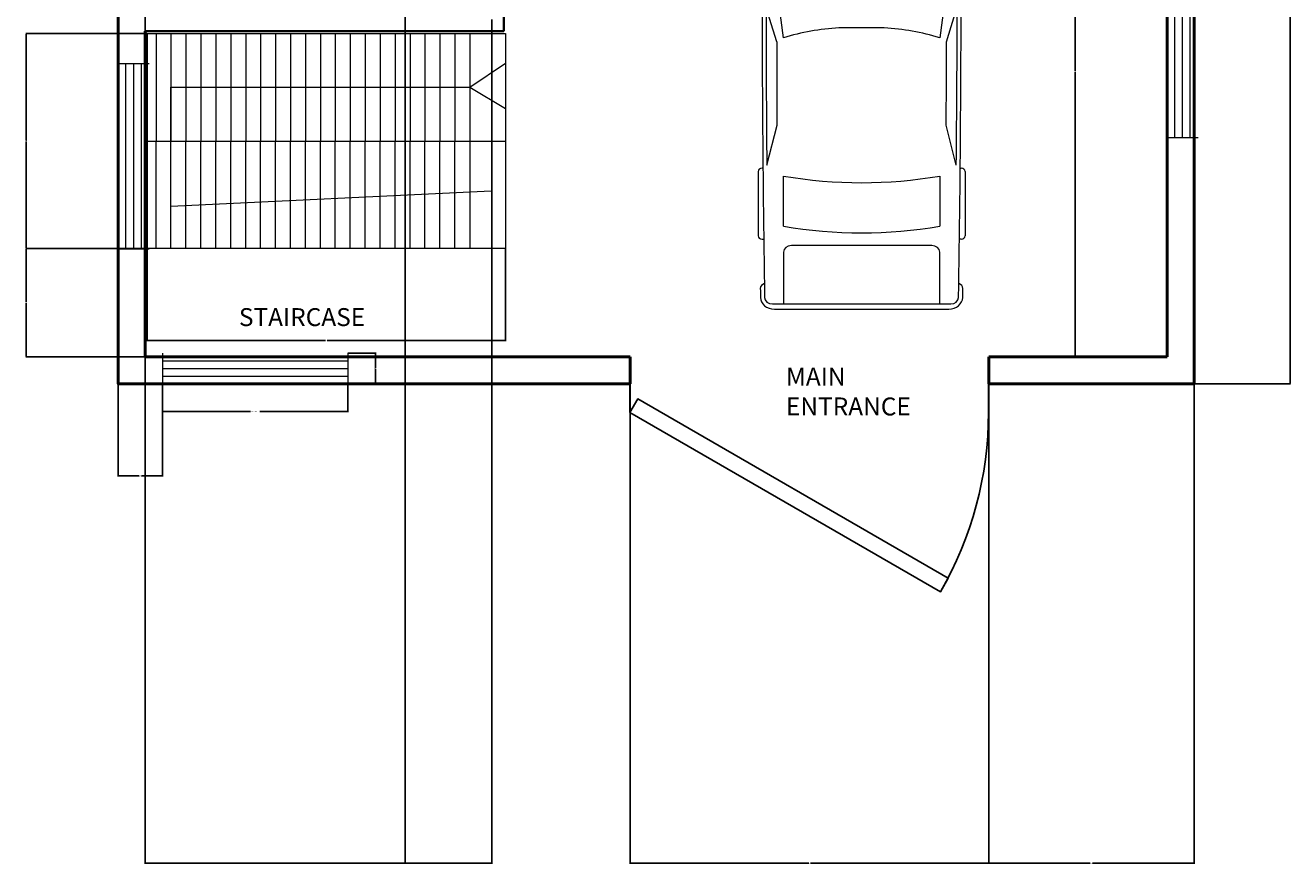
# Model space of a CAD drawing. Units: feet. Extents: x 3746 to 4170, y 1475 to 2148.
# Tile 1 of 5: x 3746 to 4170, y 1475 to 1755. Entities that reach past the tile are written whole.
import ezdxf

# ---------------------------------------------------------------- set-up
doc = ezdxf.new("R2010")
doc.units = ezdxf.units.FT
for name, color, linetype, lineweight in [('A-ANNO-DIMS', 2, 'Continuous', 18), ('A-AREA-IDEN', 7, 'Continuous', 25), ('A-FLOR-STRS', 7, 'Continuous', 18), ('A-GLAZ', 91, 'Continuous', 18), ('CAR', 20, 'Continuous', 13), ('DOOR', 135, 'Continuous', 25), ('INWER WALL', 30, 'Continuous', 35), ('OUTER WALL', 31, 'Continuous', 50)]:
    doc.layers.add(name, color=color, linetype=linetype, lineweight=lineweight)
doc.styles.get("Standard").update_dxf_attribs({"font": 'arial.ttf'})
doc.dimstyles.get("Standard").update_dxf_attribs({"dimtxt": 0.18, "dimasz": 0.18, "dimexe": 0.18, "dimexo": 0.0625, "dimgap": 0.09, "dimtad": 0, "dimtih": 1, "dimtoh": 1, "dimdec": 4, "dimzin": 0, "dimdsep": 46, "dimtxsty": 'Standard', "dimcen": 0.09, "dimadec": 0, "dimazin": 0, "dimtfac": 1, "dimtdec": 4, "dimtofl": 0, "dimtmove": 0, "dimatfit": 3, "dimfxl": 1, "dimtolj": 1, "dimtzin": 0, "dimarcsym": 0})

# ---------------------------------------------------------------- blocks, each defined once
blk = doc.blocks.new('*U12')
for p, q in [((46.55, 38.89), (22.35, 38.89)), ((136.7, 38.89), (160.9, 38.89)), ((21.1, 37.41), (21.1, 36.83)), ((47.8, 37.39), (47.8, 37.41)), ((87.99, 31.87), (74.76, 35.92)), ((134.31, 35.6), (119.29, 31.78)), ((135.45, 37.07), (135.45, 37.41)), ((162.15, 37.41), (162.15, 36.77)), ((186.47, -33.5), (186.47, 33.5)), ((70.03, 31.54), (86.41, 29.35)), ((138.42, 29.35), (157.25, 29.35)), ((186.47, 29.35), (167.01, 29.35)), ((188.4, -32.76), (188.4, 32.76)), ((164.52, 26.39), (164.52, -26.39)), ((32.27, 11.63), (36.13, 17.17)), ((36.13, 17.17), (50.94, 17.17)), ((32.12, 9.51), (32.12, 11.15)), ((58.92, -10.77), (58.92, 10.77)), ((66.55, -10.53), (66.55, 10.53)), ((186.47, -10.53), (186.47, 10.53)), ((3.27, 6.13), (0.1, 0.41)), ((29.77, 9.51), (51.68, 9.51)), ((82.74, 8.5), (82.74, -8.5)), ((0, 0), (51.68, 0)), ((0.1, -0.41), (3.27, -6.13)), ((29.77, -9.51), (51.68, -9.51)), ((32.12, -9.51), (32.12, -11.15)), ((32.27, -11.63), (36.13, -17.17)), ((36.13, -17.17), (50.94, -17.17)), ((86.41, -29.35), (70.03, -31.54)), ((87.99, -31.87), (74.76, -35.92)), ((134.31, -35.6), (119.29, -31.78)), ((157.25, -29.35), (138.42, -29.35)), ((167.01, -29.35), (186.47, -29.35)), ((21.1, -37.41), (21.1, -36.83)), ((47.8, -37.39), (47.8, -37.41)), ((135.45, -37.07), (135.45, -37.41)), ((162.15, -37.41), (162.15, -36.77)), ((46.55, -38.89), (22.35, -38.89)), ((136.7, -38.89), (160.9, -38.89))]:
    blk.add_line(p, q)
for centre, major_axis, ratio, start_param, end_param in [((22.35, 37.41), (0, -1.48), 0.842304, 3.141593, 4.712389), ((46.55, 37.41), (0, 1.48), 0.842304, -1.570796, 0), ((136.7, 37.41), (0, -1.48), 0.842304, 3.141593, 4.712389), ((160.9, 37.41), (0, 1.48), 0.842304, -1.570796, 0), ((180.63, 35.84), (0, 2.22), 0.842304, -0.013017, 1.249894), ((64.48, -10556.36), (0, 10595.31), 0.842304, -0.013397, -0.013017), ((266.03, -27.52), (0, 313.31), 0.842304, 1.367076, 1.39176), ((41.19, -490.86), (0, 528.23), 0.842304, 0.00281, 0.075598), ((64.48, -10555.62), (0, 10593.03), 0.842304, -0.013397, 0.002797), ((64.48, -10555.62), (0, -10591.55), 0.842304, 3.133765, 3.140441), ((183.98, 33.5), (0, -2.96), 0.842304, 1.570796, 3.128196), ((183.98, 32.76), (0, -5.25), 0.842304, 1.570796, 3.128196), ((37.47, -593.96), (0, -623.33), 0.842304, 3.096046, 3.200911), ((134.4, 5.39), (0, -89.78), 0.842304, 4.449482, 4.652344), ((135.29, 5.39), (0, 81.77), 0.842304, 1.245306, 1.50788), ((149.6, 2.8), (0, -79.58), 0.842304, 4.372215, 4.640744), ((95.79, -3666.35), (0, -3698.24), 0.842304, 3.134049, 3.144098), ((17.08, 0), (0, 147.02), 0.842304, 4.511394, 4.913384), ((35.91, 0), (0, 147.02), 0.842304, 4.511394, 4.913384), ((167.01, 26.39), (0, 2.96), 0.842304, 0, 1.570796), ((259.18, -27.52), (0, -305.3), 0.842304, 4.528606, 4.561838), ((-204.49, 52.4), (0, -250.96), 0.842304, 1.385369, 1.434372), ((13.04, 17.01), (0, 27.42), 0.842304, 4.435146, 4.718221), ((14.2, 17.01), (0, 27.42), 0.842304, 4.435146, 4.718221), ((50.79, 13.34), (6.34, -0.36), 0.603834, -1.395552, 1.581315), ((32.75, 11.15), (0, 0.74), 0.842304, 0.879714, 1.570796), ((29.77, -46.66), (0, 56.17), 0.842304, 0, 0.590319), ((0.62, 0), (0, -0.74), 0.842304, 4.131459, 5.293319), ((29.77, 46.66), (0, 56.17), 0.842304, 2.551274, 3.141593), ((-204.49, -52.4), (0, 250.96), 0.842304, -1.434372, -1.385369), ((13.04, -17.01), (0, -27.42), 0.842304, 1.564964, 1.848039), ((14.2, -17.01), (0, -27.42), 0.842304, 1.564964, 1.848039), ((149.6, -2.8), (0, -79.58), 0.842304, -1.499151, -1.230623), ((32.75, -11.15), (0, -0.74), 0.842304, 4.712389, 5.403472), ((134.4, -5.39), (0, -89.78), 0.842304, -1.510751, -1.307889), ((135.29, -5.39), (0, -81.77), 0.842304, -1.50788, -1.245306), ((259.18, 27.52), (0, 305.3), 0.842304, 1.721348, 1.754579), ((266.03, 27.52), (0, 313.31), 0.842304, 1.749832, 1.774517), ((37.47, 593.96), (0, -623.33), 0.842304, -0.059319, 0.045547), ((167.01, -26.39), (0, -2.96), 0.842304, 4.712389, 6.283185), ((95.79, 3666.35), (0, -3698.24), 0.842304, -0.002505, 0.007544), ((183.98, -32.76), (0, -5.25), 0.842304, 0.013397, 1.570796), ((41.19, 490.86), (0, -528.23), 0.842304, -0.075598, -0.00281), ((22.35, -37.41), (0, 1.48), 0.842304, 1.570796, 3.141593), ((64.48, 10555.62), (0, 10593.03), 0.842304, 3.138796, 3.15499), ((46.55, -37.41), (0, -1.48), 0.842304, 0, 1.570796), ((64.48, 10555.62), (0, -10591.55), 0.842304, 0.001152, 0.007828), ((136.7, -37.41), (0, -1.48), 0.842304, -1.570796, 0), ((160.9, -37.41), (0, 1.48), 0.842304, 3.141593, 4.712389), ((180.63, -35.84), (0, -2.22), 0.842304, -1.249894, 0.013017), ((64.48, 10556.36), (0, 10595.31), 0.842304, 3.15461, 3.15499), ((183.98, -33.5), (0, 2.96), 0.842304, 3.15499, 4.712389)]:
    blk.add_ellipse(centre, major_axis=major_axis, ratio=ratio, start_param=start_param, end_param=end_param)
at = {"extrusion": (0, 0, -1)}
blk.add_ellipse((50.79, -13.34), major_axis=(6.34, 0.36), ratio=0.603834, start_param=-1.395552, end_param=1.581315, dxfattribs=at)
blk = doc.blocks.new('*U3')
for p, q in [((0, 0), (0, 6)), ((40, 0), (40, 6))]:
    blk.add_line(p, q)
blk.add_lwpolyline([(0, 0), (34.64, -20), (35.52, -18.48), (0.87, 1.52)], close=True)
blk.add_arc((0, 0), 40, 330, 0)
blk = doc.blocks.new('Window - Wood Frame 36 in. Wide plan')
for p, q in [((0, 6), (0, 0)), ((36, 6), (36, 0)), ((0, 4.5), (36, 4.5)), ((0, 3), (36, 3)), ((0, 1.5), (36, 1.5))]:
    blk.add_line(p, q)
blk = doc.blocks.new('*D37')
at = {"layer": 'A-ANNO-DIMS', "color": 0, "lineweight": -2, "transparency": 16777216}
for p, q in [((3792.26, 1635.32), (3792.26, 1625.91)), ((3854.23, 1635.32), (3854.23, 1625.91)), ((3792.44, 1626.09), (3821.69, 1626.09)), ((3854.05, 1626.09), (3824.8, 1626.09))]:
    blk.add_line(p, q, dxfattribs=at)
at = {"layer": 'A-ANNO-DIMS', "color": 0, "transparency": 16777216}
for points in [[(3792.44, 1626.12), (3792.44, 1626.06), (3792.26, 1626.09)], [(3854.05, 1626.12), (3854.05, 1626.06), (3854.23, 1626.09)]]:
    blk.add_solid(points, dxfattribs=at)
at = {"layer": 'Defpoints', "color": 0, "transparency": 16777216}
for p in [(3792.26, 1635.38), (3854.23, 1635.38), (3854.23, 1626.09)]:
    blk.add_point(p, dxfattribs=at)
at = {"layer": 'A-ANNO-DIMS', "color": 0, "transparency": 16777216, "insert": (3823.24, 1626.09), "char_height": 0.18, "attachment_point": 5}
blk.add_mtext('\\A1;WOOD WINDOW 62 TYP.', dxfattribs=at)
blk = doc.blocks.new('*D38')
at = {"layer": 'A-ANNO-DIMS', "color": 0, "lineweight": -2, "transparency": 16777216}
for p, q in [((3854.29, 1645.71), (3863.7, 1645.71)), ((3863.52, 1645.53), (3863.52, 1640.73)), ((3863.52, 1635.56), (3863.52, 1640.36)), ((3854.29, 1635.38), (3863.7, 1635.38))]:
    blk.add_line(p, q, dxfattribs=at)
at = {"layer": 'A-ANNO-DIMS', "color": 0, "transparency": 16777216}
for points in [[(3863.49, 1645.53), (3863.55, 1645.53), (3863.52, 1645.71)], [(3863.49, 1635.56), (3863.55, 1635.56), (3863.52, 1635.38)]]:
    blk.add_solid(points, dxfattribs=at)
at = {"layer": 'Defpoints', "color": 0, "transparency": 16777216}
for p in [(3854.23, 1645.71), (3863.52, 1645.71), (3854.23, 1635.38)]:
    blk.add_point(p, dxfattribs=at)
at = {"layer": 'A-ANNO-DIMS', "color": 0, "transparency": 16777216, "insert": (3863.52, 1640.55), "char_height": 0.18, "attachment_point": 5}
blk.add_mtext('\\A1;10 TYP.', dxfattribs=at)
blk = doc.blocks.new('*D56')
at = {"layer": 'A-ANNO-DIMS', "color": 0, "lineweight": -2, "transparency": 16777216}
for p, q in [((4137.49, 2115.38), (4169.74, 2115.38)), ((4169.56, 2115.2), (4169.56, 1875.56)), ((4169.56, 1635.56), (4169.56, 1875.2)), ((4137.49, 1635.38), (4169.74, 1635.38))]:
    blk.add_line(p, q, dxfattribs=at)
at = {"layer": 'A-ANNO-DIMS', "color": 0, "transparency": 16777216}
for points in [[(4169.53, 2115.2), (4169.59, 2115.2), (4169.56, 2115.38)], [(4169.53, 1635.56), (4169.59, 1635.56), (4169.56, 1635.38)]]:
    blk.add_solid(points, dxfattribs=at)
at = {"layer": 'Defpoints', "color": 0, "transparency": 16777216}
for p in [(4137.43, 2115.38), (4137.43, 1635.38), (4169.56, 1635.38)]:
    blk.add_point(p, dxfattribs=at)
at = {"layer": 'A-ANNO-DIMS', "color": 0, "transparency": 16777216, "insert": (4169.56, 1875.38), "char_height": 0.18, "attachment_point": 5}
blk.add_mtext('\\A1;480', dxfattribs=at)
blk = doc.blocks.new('*D63')
at = {"layer": 'A-ANNO-DIMS', "color": 0, "lineweight": -2, "transparency": 16777216}
for p, q in [((3786.43, 1970.32), (3786.43, 1474.8)), ((3873.43, 1922.32), (3873.43, 1474.8)), ((3786.61, 1474.98), (3829.71, 1474.98)), ((3873.25, 1474.98), (3830.15, 1474.98))]:
    blk.add_line(p, q, dxfattribs=at)
at = {"layer": 'A-ANNO-DIMS', "color": 0, "transparency": 16777216}
for points in [[(3786.61, 1475.01), (3786.61, 1474.95), (3786.43, 1474.98)], [(3873.25, 1475.01), (3873.25, 1474.95), (3873.43, 1474.98)]]:
    blk.add_solid(points, dxfattribs=at)
at = {"layer": 'Defpoints', "color": 0, "transparency": 16777216}
for p in [(3786.43, 1970.38), (3873.43, 1922.38), (3873.43, 1474.98)]:
    blk.add_point(p, dxfattribs=at)
at = {"layer": 'A-ANNO-DIMS', "color": 0, "transparency": 16777216, "insert": (3829.93, 1474.98), "char_height": 0.18, "attachment_point": 5}
blk.add_mtext('\\A1;87', dxfattribs=at)
blk = doc.blocks.new('*D68')
at = {"layer": 'A-ANNO-DIMS', "color": 0, "lineweight": -2, "transparency": 16777216}
for p, q in [((3786.43, 1757.32), (3786.43, 1474.8)), ((3902.43, 1757.32), (3902.43, 1474.8)), ((3786.61, 1474.98), (3844.15, 1474.98)), ((3902.25, 1474.98), (3844.71, 1474.98))]:
    blk.add_line(p, q, dxfattribs=at)
at = {"layer": 'A-ANNO-DIMS', "color": 0, "transparency": 16777216}
for points in [[(3786.61, 1475.01), (3786.61, 1474.95), (3786.43, 1474.98)], [(3902.25, 1475.01), (3902.25, 1474.95), (3902.43, 1474.98)]]:
    blk.add_solid(points, dxfattribs=at)
at = {"layer": 'Defpoints', "color": 0, "transparency": 16777216}
for p in [(3786.43, 1757.38), (3902.43, 1757.38), (3902.43, 1474.98)]:
    blk.add_point(p, dxfattribs=at)
at = {"layer": 'A-ANNO-DIMS', "color": 0, "transparency": 16777216, "insert": (3844.43, 1474.98), "char_height": 0.18, "attachment_point": 5}
blk.add_mtext('\\A1;116', dxfattribs=at)
blk = doc.blocks.new('*D72')
at = {"layer": 'A-ANNO-DIMS', "color": 0, "lineweight": -2, "transparency": 16777216}
for p, q in [((4128.37, 1835.38), (4097.45, 1835.38)), ((4097.63, 1835.2), (4097.63, 1740.06)), ((4097.63, 1644.56), (4097.63, 1739.7)), ((4128.37, 1644.38), (4097.45, 1644.38))]:
    blk.add_line(p, q, dxfattribs=at)
at = {"layer": 'A-ANNO-DIMS', "color": 0, "transparency": 16777216}
for points in [[(4097.6, 1835.2), (4097.66, 1835.2), (4097.63, 1835.38)], [(4097.6, 1644.56), (4097.66, 1644.56), (4097.63, 1644.38)]]:
    blk.add_solid(points, dxfattribs=at)
at = {"layer": 'Defpoints', "color": 0, "transparency": 16777216}
for p in [(4097.63, 1835.38), (4128.43, 1835.38), (4128.43, 1644.38)]:
    blk.add_point(p, dxfattribs=at)
at = {"layer": 'A-ANNO-DIMS', "color": 0, "transparency": 16777216, "insert": (4097.63, 1739.88), "char_height": 0.18, "attachment_point": 5}
blk.add_mtext('\\A1;191', dxfattribs=at)
blk = doc.blocks.new('*D73')
at = {"layer": 'A-ANNO-DIMS', "color": 0, "lineweight": -2, "transparency": 16777216}
for p, q in [((3787, 1752.65), (3746.45, 1752.65)), ((3746.63, 1752.47), (3746.63, 1716.83)), ((3746.63, 1680.83), (3746.63, 1716.47)), ((3787, 1680.65), (3746.45, 1680.65))]:
    blk.add_line(p, q, dxfattribs=at)
at = {"layer": 'A-ANNO-DIMS', "color": 0, "transparency": 16777216}
for points in [[(3746.6, 1752.47), (3746.66, 1752.47), (3746.63, 1752.65)], [(3746.6, 1680.83), (3746.66, 1680.83), (3746.63, 1680.65)]]:
    blk.add_solid(points, dxfattribs=at)
at = {"layer": 'Defpoints', "color": 0, "transparency": 16777216}
for p in [(3787.06, 1752.65), (3746.63, 1680.65), (3787.06, 1680.65)]:
    blk.add_point(p, dxfattribs=at)
at = {"layer": 'A-ANNO-DIMS', "color": 0, "transparency": 16777216, "insert": (3746.63, 1716.65), "char_height": 0.18, "attachment_point": 5}
blk.add_mtext('\\A1;72', dxfattribs=at)
blk = doc.blocks.new('*D74')
at = {"layer": 'A-ANNO-DIMS', "color": 0, "lineweight": -2, "transparency": 16777216}
for p, q in [((3787, 1680.65), (3746.45, 1680.65)), ((3746.63, 1680.47), (3746.63, 1662.7)), ((3746.63, 1644.56), (3746.63, 1662.34)), ((3786.37, 1644.38), (3746.45, 1644.38))]:
    blk.add_line(p, q, dxfattribs=at)
at = {"layer": 'A-ANNO-DIMS', "color": 0, "transparency": 16777216}
for points in [[(3746.6, 1680.47), (3746.66, 1680.47), (3746.63, 1680.65)], [(3746.6, 1644.56), (3746.66, 1644.56), (3746.63, 1644.38)]]:
    blk.add_solid(points, dxfattribs=at)
at = {"layer": 'Defpoints', "color": 0, "transparency": 16777216}
for p in [(3787.06, 1680.65), (3746.63, 1644.38), (3786.43, 1644.38)]:
    blk.add_point(p, dxfattribs=at)
at = {"layer": 'A-ANNO-DIMS', "color": 0, "transparency": 16777216, "insert": (3746.63, 1662.52), "char_height": 0.18, "attachment_point": 5}
blk.add_mtext('\\A1;36.27', dxfattribs=at)
blk = doc.blocks.new('*D75')
at = {"layer": 'A-ANNO-DIMS', "color": 0, "lineweight": -2, "transparency": 16777216}
for p, q in [((3948.75, 1635.32), (3948.75, 1474.8)), ((4068.75, 1635.32), (4068.75, 1474.8)), ((3948.93, 1474.98), (4008.47, 1474.98)), ((4068.57, 1474.98), (4009.03, 1474.98))]:
    blk.add_line(p, q, dxfattribs=at)
at = {"layer": 'A-ANNO-DIMS', "color": 0, "transparency": 16777216}
for points in [[(3948.93, 1475.01), (3948.93, 1474.95), (3948.75, 1474.98)], [(4068.57, 1475.01), (4068.57, 1474.95), (4068.75, 1474.98)]]:
    blk.add_solid(points, dxfattribs=at)
at = {"layer": 'Defpoints', "color": 0, "transparency": 16777216}
for p in [(3948.75, 1635.38), (4068.75, 1635.38), (4068.75, 1474.98)]:
    blk.add_point(p, dxfattribs=at)
at = {"layer": 'A-ANNO-DIMS', "color": 0, "transparency": 16777216, "insert": (4008.75, 1474.98), "char_height": 0.18, "attachment_point": 5}
blk.add_mtext('\\A1;120', dxfattribs=at)
blk = doc.blocks.new('*D76')
at = {"layer": 'A-ANNO-DIMS', "color": 0, "lineweight": -2, "transparency": 16777216}
for p, q in [((4068.75, 1635.32), (4068.75, 1474.8)), ((4137.43, 1635.32), (4137.43, 1474.8)), ((4068.93, 1474.98), (4102.7, 1474.98)), ((4137.25, 1474.98), (4103.49, 1474.98))]:
    blk.add_line(p, q, dxfattribs=at)
at = {"layer": 'A-ANNO-DIMS', "color": 0, "transparency": 16777216}
for points in [[(4068.93, 1475.01), (4068.93, 1474.95), (4068.75, 1474.98)], [(4137.25, 1475.01), (4137.25, 1474.95), (4137.43, 1474.98)]]:
    blk.add_solid(points, dxfattribs=at)
at = {"layer": 'Defpoints', "color": 0, "transparency": 16777216}
for p in [(4068.75, 1635.38), (4137.43, 1635.38), (4137.43, 1474.98)]:
    blk.add_point(p, dxfattribs=at)
at = {"layer": 'A-ANNO-DIMS', "color": 0, "transparency": 16777216, "insert": (4103.09, 1474.98), "char_height": 0.18, "attachment_point": 5}
blk.add_mtext('\\A1;68.68', dxfattribs=at)
blk = doc.blocks.new('*D86')
at = {"layer": 'A-ANNO-DIMS', "color": 0, "lineweight": -2, "transparency": 16777216}
for p, q in [((3777.43, 1635.32), (3777.43, 1604.4)), ((3792.26, 1635.32), (3792.26, 1604.4)), ((3777.61, 1604.58), (3784.46, 1604.58)), ((3792.08, 1604.58), (3785.23, 1604.58))]:
    blk.add_line(p, q, dxfattribs=at)
at = {"layer": 'A-ANNO-DIMS', "color": 0, "transparency": 16777216}
for points in [[(3777.61, 1604.61), (3777.61, 1604.55), (3777.43, 1604.58)], [(3792.08, 1604.61), (3792.08, 1604.55), (3792.26, 1604.58)]]:
    blk.add_solid(points, dxfattribs=at)
at = {"layer": 'Defpoints', "color": 0, "transparency": 16777216}
for p in [(3777.43, 1635.38), (3792.26, 1635.38), (3777.43, 1604.58)]:
    blk.add_point(p, dxfattribs=at)
at = {"layer": 'A-ANNO-DIMS', "color": 0, "transparency": 16777216, "insert": (3784.84, 1604.58), "char_height": 0.18, "attachment_point": 5}
blk.add_mtext('\\A1;14.83', dxfattribs=at)
blk = doc.blocks.new('*D88')
at = {"layer": 'A-ANNO-DIMS', "color": 0, "lineweight": -2, "transparency": 16777216}
for p, q in [((3787.06, 1680.59), (3787.06, 1649.67)), ((3907.06, 1680.59), (3907.06, 1649.67)), ((3787.24, 1649.85), (3846.78, 1649.85)), ((3906.88, 1649.85), (3847.34, 1649.85))]:
    blk.add_line(p, q, dxfattribs=at)
at = {"layer": 'A-ANNO-DIMS', "color": 0, "transparency": 16777216}
for points in [[(3787.24, 1649.88), (3787.24, 1649.82), (3787.06, 1649.85)], [(3906.88, 1649.88), (3906.88, 1649.82), (3907.06, 1649.85)]]:
    blk.add_solid(points, dxfattribs=at)
at = {"layer": 'Defpoints', "color": 0, "transparency": 16777216}
for p in [(3787.06, 1680.65), (3907.06, 1680.65), (3787.06, 1649.85)]:
    blk.add_point(p, dxfattribs=at)
at = {"layer": 'A-ANNO-DIMS', "color": 0, "transparency": 16777216, "insert": (3847.06, 1649.85), "char_height": 0.18, "attachment_point": 5}
blk.add_mtext('\\A1;120', dxfattribs=at)

msp = doc.modelspace()

# ---------------------------------------------------------------- linework, layer by layer
at = {"layer": 'A-FLOR-STRS'}
for p, q in [((3787.0644, 1752.6518), (3907.0644, 1752.6518)), ((3787.0644, 1680.6518), (3787.0644, 1752.6518)), ((3787.0644, 1752.6518), (3787.0644, 1752.6518)), ((3787.0644, 1752.6518), (3787.0644, 1680.6518)), ((3790.0644, 1752.6518), (3790.0644, 1716.6518)), ((3795.0644, 1752.6518), (3795.0644, 1716.6518)), ((3800.0644, 1752.6518), (3800.0644, 1716.6518)), ((3805.0644, 1752.6518), (3805.0644, 1716.6518)), ((3810.0644, 1752.6518), (3810.0644, 1716.6518)), ((3815.0644, 1752.6518), (3815.0644, 1716.6518)), ((3820.0644, 1752.6518), (3820.0644, 1716.6518)), ((3825.0644, 1752.6518), (3825.0644, 1716.6518)), ((3830.0644, 1752.6518), (3830.0644, 1716.6518)), ((3835.0644, 1752.6518), (3835.0644, 1716.6518)), ((3840.0644, 1752.6518), (3840.0644, 1716.6518)), ((3845.0644, 1752.6518), (3845.0644, 1716.6518)), ((3850.0644, 1752.6518), (3850.0644, 1716.6518)), ((3855.0644, 1752.6518), (3855.0644, 1716.6518)), ((3860.0644, 1752.6518), (3860.0644, 1716.6518)), ((3865.0644, 1752.6518), (3865.0644, 1716.6518)), ((3870.0644, 1752.6518), (3870.0644, 1716.6518)), ((3875.0644, 1752.6518), (3875.0644, 1716.6518)), ((3880.0644, 1752.6518), (3880.0644, 1716.6518)), ((3885.0644, 1752.6518), (3885.0644, 1716.6518)), ((3890.0644, 1752.6518), (3890.0644, 1716.6518)), ((3895.0644, 1752.6518), (3895.0644, 1716.6518)), ((3907.0644, 1752.6518), (3907.0644, 1716.6518)), ((3895.0644, 1734.6518), (3907.0644, 1742.7393)), ((3795.0644, 1694.7821), (3795.0644, 1734.6518)), ((3795.0644, 1734.6518), (3895.0644, 1734.6518)), ((3895.0644, 1734.6518), (3907.0644, 1727.5645)), ((3787.0644, 1716.6518), (3907.0644, 1716.6518)), ((3790.0644, 1680.6518), (3790.0644, 1716.6518)), ((3795.0644, 1680.6518), (3795.0644, 1716.6518)), ((3800.0644, 1680.6518), (3800.0644, 1716.6518)), ((3805.0644, 1680.6518), (3805.0644, 1716.6518)), ((3810.0644, 1680.6518), (3810.0644, 1716.6518)), ((3815.0644, 1680.6518), (3815.0644, 1716.6518)), ((3820.0644, 1680.6518), (3820.0644, 1716.6518)), ((3825.0644, 1680.6518), (3825.0644, 1716.6518)), ((3830.0644, 1680.6518), (3830.0644, 1716.6518)), ((3835.0644, 1680.6518), (3835.0644, 1716.6518)), ((3840.0644, 1680.6518), (3840.0644, 1716.6518)), ((3845.0644, 1680.6518), (3845.0644, 1716.6518)), ((3850.0644, 1680.6518), (3850.0644, 1716.6518)), ((3855.0644, 1680.6518), (3855.0644, 1716.6518)), ((3860.0644, 1680.6518), (3860.0644, 1716.6518)), ((3865.0644, 1680.6518), (3865.0644, 1716.6518)), ((3870.0644, 1680.6518), (3870.0644, 1716.6518)), ((3875.0644, 1680.6518), (3875.0644, 1716.6518)), ((3880.0644, 1680.6518), (3880.0644, 1716.6518)), ((3885.0644, 1680.6518), (3885.0644, 1716.6518)), ((3890.0644, 1680.6518), (3890.0644, 1716.6518)), ((3895.0644, 1716.6518), (3895.0644, 1680.6518)), ((3907.0644, 1716.6518), (3907.0644, 1680.6518)), ((3902.2562, 1699.869), (3795.0644, 1694.7821)), ((3907.0644, 1680.6518), (3787.0644, 1680.6518)), ((3787.0644, 1680.6518), (3787.0644, 1680.6518))]:
    msp.add_line(p, q, dxfattribs=at)
at = {"layer": 'INWER WALL'}
for p, q in [((3906.4289, 1753.3828), (3906.4289, 1835.3828)), ((3786.4289, 1753.3828), (3906.4289, 1753.3828))]:
    msp.add_line(p, q, dxfattribs=at)
at = {"layer": 'OUTER WALL'}
for p, q in [((4128.4289, 1835.3828), (4128.4289, 1644.3828)), ((3786.4289, 1644.3828), (3786.4289, 1753.3828)), ((3948.7526, 1644.3828), (3786.4289, 1644.3828)), ((3948.7526, 1644.3828), (3948.7526, 1635.3828)), ((4128.4289, 1644.3828), (4068.7526, 1644.3828)), ((4068.7526, 1644.3828), (4068.7526, 1635.3828))]:
    msp.add_line(p, q, dxfattribs=at)
msp.add_lwpolyline([(3948.7526, 1635.3828), (3777.4289, 1635.3828), (3777.4289, 2115.3828), (4137.4289, 2115.3828), (4137.4289, 1635.3828), (4068.7526, 1635.3828)], dxfattribs=at)

# ---------------------------------------------------------------- block references
at = {"layer": 'A-GLAZ', "xscale": 1.721338572628536, "yscale": 1.721338572628536, "zscale": 1.721338572628536, "rotation": 90}
for p in [(4138.7569, 1717.8058), (3787.7569, 1680.5978)]:
    msp.add_blockref('Window - Wood Frame 36 in. Wide plan', p, dxfattribs=at)
at = {"layer": 'A-GLAZ', "xscale": 1.721338572628536, "yscale": 1.721338572628536, "zscale": 1.721338572628536}
msp.add_blockref('Window - Wood Frame 36 in. Wide plan', (3792.2599, 1635.3828), dxfattribs=at)
at = {"layer": 'CAR', "xscale": 0.890498965628364, "yscale": 0.890498965628364, "zscale": 0.890498965628364, "rotation": 270}
msp.add_blockref('*U12', (4026.167, 1828.1892), dxfattribs=at)
at = {"layer": 'DOOR', "xscale": 3.000000000000029, "yscale": 3.000000000000029, "zscale": 3.000000000000029}
msp.add_blockref('*U3', (3948.6302, 1625.78), dxfattribs=at)

# ---------------------------------------------------------------- texts
at = {"layer": 'A-AREA-IDEN', "char_height": 6, "attachment_point": 1}
for s, insert in [('STAIRCASE', (3817.7989, 1660.7258)), ('MAIN ENTRANCE', (4000.8647, 1640.8256))]:
    msp.add_mtext_dynamic_manual_height_columns(s, width=45.721785, gutter_width=12.5, heights=[0], dxfattribs=dict(at, insert=insert))

# ---------------------------------------------------------------- dimensions: what is measured, and where the dimension line sits
at = {"layer": 'A-ANNO-DIMS'}
for base, p1, p2, angle, override, picture, middle in [((4169.5569, 1635.3828), (4137.4289, 2115.3828), (4137.4289, 1635.3828), 90, {"dimdec": 0, "dimlfac": 1, "dimrnd": 0, "dimzin": 0, "dimdsep": 46, "dimlunit": 2}, '*D56', (4169.5569, 1875.3828)), ((4097.6289, 1835.3828), (4128.4289, 1644.3828), (4128.4289, 1835.3828), 90, {"dimdec": 0, "dimlfac": 1, "dimrnd": 0, "dimzin": 0, "dimdsep": 46, "dimlunit": 2}, '*D72', (4097.6289, 1739.8828)), ((3746.6289, 1680.6518), (3787.0644, 1752.6518), (3787.0644, 1680.6518), 90, {"dimdec": 0, "dimlfac": 1, "dimrnd": 0, "dimzin": 0, "dimdsep": 46, "dimlunit": 2}, '*D73', (3746.6289, 1716.6518)), ((3746.6289, 1644.3828), (3787.0644, 1680.6518), (3786.4289, 1644.3828), 90, {"dimdec": 2, "dimlfac": 1, "dimrnd": 0, "dimzin": 0, "dimdsep": 46, "dimlunit": 2}, '*D74', (3746.6289, 1662.5173)), ((3787.0644, 1649.8518), (3907.0644, 1680.6518), (3787.0644, 1680.6518), 180, {"dimdec": 0, "dimlfac": 1, "dimrnd": 0, "dimzin": 0, "dimdsep": 46, "dimlunit": 2}, '*D88', (3847.0644, 1649.8518)), ((3777.4289, 1604.5828), (3792.2599, 1635.3828), (3777.4289, 1635.3828), 180, {"dimdec": 2, "dimlfac": 1, "dimrnd": 0, "dimzin": 0, "dimdsep": 46, "dimlunit": 2}, '*D86', (3784.8444, 1604.5828))]:
    dim = msp.add_linear_dim(base=base, p1=p1, p2=p2, angle=angle, dimstyle='Standard', override=override, dxfattribs=at)
    dim.commit()
    dim.dimension.update_dxf_attribs({"geometry": picture, "text_midpoint": middle})
for base, p1, p2, override, picture, middle in [((3873.4289, 1474.98), (3786.4289, 1970.3828), (3873.4289, 1922.3828), {"dimdec": 0, "dimlfac": 1, "dimrnd": 0, "dimzin": 0, "dimdsep": 46, "dimlunit": 2}, '*D63', (3829.9289, 1474.98)), ((3902.4289, 1474.98), (3786.4289, 1757.3828), (3902.4289, 1757.3828), {"dimdec": 0, "dimlfac": 1, "dimrnd": 0, "dimzin": 0, "dimdsep": 46, "dimlunit": 2}, '*D68', (3844.4289, 1474.98)), ((4068.7526, 1474.98), (3948.7526, 1635.3828), (4068.7526, 1635.3828), {"dimdec": 0, "dimlfac": 1, "dimrnd": 0, "dimzin": 0, "dimdsep": 46, "dimlunit": 2}, '*D75', (4008.7526, 1474.98)), ((4137.4289, 1474.98), (4068.7526, 1635.3828), (4137.4289, 1635.3828), {"dimdec": 2, "dimlfac": 1, "dimrnd": 0, "dimzin": 0, "dimdsep": 46, "dimlunit": 2}, '*D76', (4103.0907, 1474.98))]:
    dim = msp.add_linear_dim(base=base, p1=p1, p2=p2, dimstyle='Standard', override=override, dxfattribs=at)
    dim.commit()
    dim.dimension.update_dxf_attribs({"geometry": picture, "text_midpoint": middle})
dim = msp.add_linear_dim(base=(3863.5233, 1645.7109), p1=(3854.2281, 1635.3828), p2=(3854.2281, 1645.7109), angle=90, text='<> TYP.', dimstyle='Standard', override={"dimdec": 0, "dimlfac": 1, "dimrnd": 0, "dimzin": 0, "dimdsep": 46, "dimlunit": 2}, dxfattribs=at)
dim.commit()
dim.dimension.update_dxf_attribs({"geometry": '*D38', "text_midpoint": (3863.5233, 1640.5468)})
dim = msp.add_linear_dim(base=(3854.2281, 1626.0876), p1=(3792.2599, 1635.3828), p2=(3854.2281, 1635.3828), text='WOOD WINDOW <> TYP.', dimstyle='Standard', override={"dimdec": 0, "dimlfac": 1, "dimrnd": 0, "dimzin": 0, "dimdsep": 46, "dimlunit": 2}, dxfattribs=at)
dim.commit()
dim.dimension.update_dxf_attribs({"geometry": '*D37', "text_midpoint": (3823.244, 1626.0876)})

doc.saveas('drawing.dxf')
